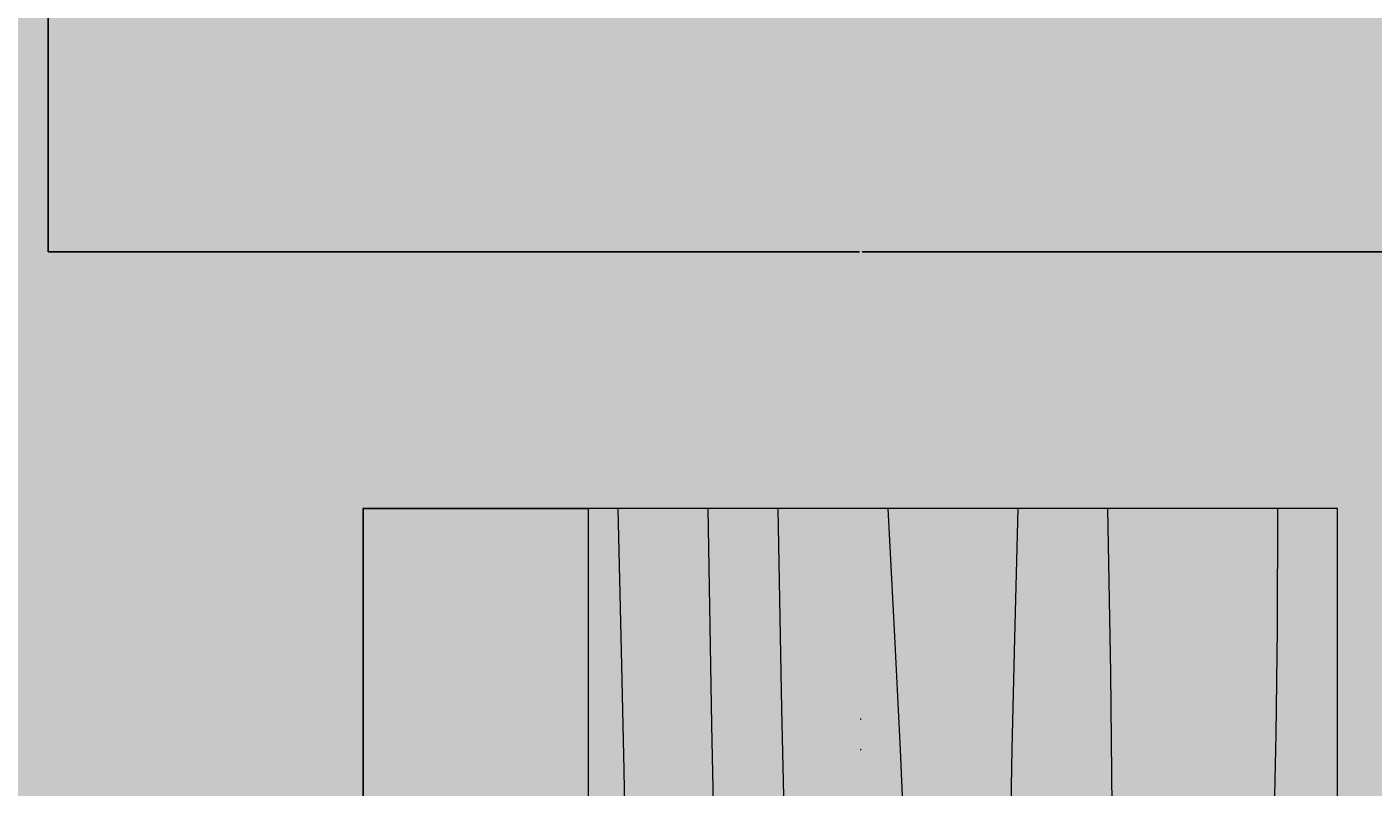
# Model space of a CAD drawing. Units: millimetres. Extents: x -229 to 16545, y -10488 to 4272.
# Tile 20 of 29: x 11572 to 12629, y -2708 to -2111. Entities that reach past the tile are written whole.
import ezdxf

# ---------------------------------------------------------------- set-up
doc = ezdxf.new("R2010")
doc.units = ezdxf.units.MM
for name, color, linetype, lineweight in [('A-ANNO-DIMS', 2, 'Continuous', 18), ('A-FURN', 8, 'Continuous', 18), ('A-FURN-PATT', 252, 'Continuous', 13)]:
    doc.layers.add(name, color=color, linetype=linetype, lineweight=lineweight)
doc.layers.add('A-FLOR-PATT', color=254, linetype='Continuous', lineweight=13, true_color=0xfeeab9)
doc.styles.get("Standard").update_dxf_attribs({"font": 'arial.ttf'})
doc.dimstyles.get("Standard").update_dxf_attribs({"dimtxt": 0.18, "dimasz": 0.18, "dimexe": 0.18, "dimexo": 0.0625, "dimgap": 0.09, "dimtad": 0, "dimtih": 1, "dimtoh": 1, "dimdec": 4, "dimzin": 0, "dimdsep": 46, "dimtxsty": 'Standard', "dimcen": 0.09, "dimadec": 0, "dimazin": 0, "dimtfac": 1, "dimtdec": 4, "dimtofl": 0, "dimtmove": 0, "dimatfit": 3, "dimfxl": 1, "dimtolj": 1, "dimtzin": 0, "dimarcsym": 0})

# ---------------------------------------------------------------- blocks, each defined once
blk = doc.blocks.new('Table - Rectangular Woodgrain 60 x 30 in.')
for p, q in [((0, 0), (0, -30)), ((60, 0), (0, 0)), ((0, -30), (60, -30))]:
    blk.add_line(p, q)
for points in [[(0, -2.4), (4.8155, -2.418), (9.0302, -2.4688), (12.709, -2.5477)], [(0, -9.2), (6.5759, -9.0858), (11.9385, -9.0365)], [(0, -12.8), (5.1847, -12.9322), (9.6213, -13.0323), (13.3963, -13.1059)], [(0, -18), (5.124, -17.7273), (9.6609, -17.5057), (13.6705, -17.3303)], [(0, -22.4), (8.0098, -22.2501), (14.4094, -22.1011)], [(0, -25.2), (8.6355, -25.0504), (15.7026, -24.9031)], [(0, -28.8), (5.6867, -28.6681), (10.45, -28.5698), (14.407, -28.5012)]]:
    blk.add_lwpolyline(points)
blk = doc.blocks.new('*D39')
at = {"layer": 'A-ANNO-DIMS', "color": 0, "lineweight": -2, "transparency": 16777216}
for p, q in [((11588.8, -2096.3), (11588.8, -2287.9)), ((12864.9, -2096.3), (12864.9, -2287.9)), ((11588.9, -2287.7), (12225.8, -2287.7)), ((12864.7, -2287.7), (12227.9, -2287.7))]:
    blk.add_line(p, q, dxfattribs=at)
at = {"layer": 'A-ANNO-DIMS', "color": 0, "transparency": 16777216}
for points in [[(11588.9, -2287.7), (11588.9, -2287.7), (11588.8, -2287.7)], [(12864.7, -2287.7), (12864.7, -2287.7), (12864.9, -2287.7)]]:
    blk.add_solid(points, dxfattribs=at)
at = {"layer": 'Defpoints', "color": 0, "transparency": 16777216}
for p in [(11588.8, -2096.3), (12864.9, -2096.3), (12864.9, -2287.7)]:
    blk.add_point(p, dxfattribs=at)
at = {"layer": 'A-ANNO-DIMS', "color": 0, "transparency": 16777216, "insert": (12226.8, -2287.7), "char_height": 0.18, "attachment_point": 5}
blk.add_mtext('\\A1;LOVESEAT 1276', dxfattribs=at)
blk = doc.blocks.new('*D41')
at = {"layer": 'A-ANNO-DIMS', "color": 0, "lineweight": -2, "transparency": 16777216}
for p, q in [((12012.6, -2489.4), (11836, -2489.4)), ((11836.2, -2489.6), (11836.2, -3077.5)), ((11836.2, -3665.8), (11836.2, -3077.9)), ((12012.6, -3666), (11836, -3666))]:
    blk.add_line(p, q, dxfattribs=at)
at = {"layer": 'A-ANNO-DIMS', "color": 0, "transparency": 16777216}
for points in [[(11836.2, -2489.6), (11836.2, -2489.6), (11836.2, -2489.4)], [(11836.2, -3665.8), (11836.2, -3665.8), (11836.2, -3666)]]:
    blk.add_solid(points, dxfattribs=at)
at = {"layer": 'Defpoints', "color": 0, "transparency": 16777216}
for p in [(12012.7, -2489.4), (11836.2, -3666), (12012.7, -3666)]:
    blk.add_point(p, dxfattribs=at)
at = {"layer": 'A-ANNO-DIMS', "color": 0, "transparency": 16777216, "insert": (11836.2, -3077.7), "char_height": 0.18, "attachment_point": 5}
blk.add_mtext('\\A1;LOW TABLE 1177', dxfattribs=at)
blk = doc.blocks.new('*D103')
at = {"layer": 'A-ANNO-DIMS', "color": 0, "lineweight": -2, "transparency": 16777216}
for p, q in [((12227, -604.2), (12226.8, -604.2)), ((12226.8, -604.2), (12226.8, -1372.9)), ((12226.7, -2654.6), (12226.9, -2654.6)), ((12226.8, -2654.7), (12226.8, -2654.5))]:
    blk.add_line(p, q, dxfattribs=at)
at = {"layer": 'A-ANNO-DIMS', "color": 0, "transparency": 16777216}
blk.add_solid([(12226.8, -1372.9), (12226.9, -1372.9), (12226.8, -1373.1)], dxfattribs=at)
at = {"layer": 'Defpoints', "color": 0, "transparency": 16777216}
for p in [(12226.8, -1373.1), (12226.8, -2654.6)]:
    blk.add_point(p, dxfattribs=at)
at = {"layer": 'A-ANNO-DIMS', "color": 0, "transparency": 16777216, "insert": (12227.6, -604.2), "char_height": 0.18, "attachment_point": 5}
blk.add_mtext('\\A1;R1281.5', dxfattribs=at)
blk = doc.blocks.new('*D104')
at = {"layer": 'A-ANNO-DIMS', "color": 0, "lineweight": -2, "transparency": 16777216}
for p, q in [((12227, -793.9), (12226.8, -793.9)), ((12226.8, -793.9), (12226.8, -1500.5)), ((12226.7, -2678.7), (12226.9, -2678.7)), ((12226.8, -2678.8), (12226.8, -2678.6))]:
    blk.add_line(p, q, dxfattribs=at)
at = {"layer": 'A-ANNO-DIMS', "color": 0, "transparency": 16777216}
blk.add_solid([(12226.8, -1500.5), (12226.9, -1500.5), (12226.8, -1500.7)], dxfattribs=at)
at = {"layer": 'Defpoints', "color": 0, "transparency": 16777216}
for p in [(12226.8, -1500.7), (12226.8, -2678.7)]:
    blk.add_point(p, dxfattribs=at)
at = {"layer": 'A-ANNO-DIMS', "color": 0, "transparency": 16777216, "insert": (12227.5, -793.9), "char_height": 0.18, "attachment_point": 5}
blk.add_mtext('\\A1;R1178', dxfattribs=at)

msp = doc.modelspace()

# ---------------------------------------------------------------- hatches: boundary and pattern name
at = {"layer": 'A-FLOR-PATT', "transparency": 33554592}
h = msp.add_hatch(color=256, dxfattribs=at)
h.dxf.hatch_style = 1
h.paths.add_polyline_path([(7975.933, -5325.772), (7943.121, -5325.772), (7943.121, -4576.49, 0.40145271), (7225.933, -5325.772, 0.40145271), (6508.746, -4576.49), (6508.746, -5325.772), (6475.933, -5325.772), (6475.933, -5438.272), (5975.933, -5438.272), (5975.933, -7267.724), (5975.933, -7438.272), (6478.619, -7438.272), (6463.448, -7355.919), (6464.88, -7356.837), (6463.849, -7358.097), (6478.619, -7438.272), (6610.327, -7438.272), (6632.656, -7409.564), (6632.525, -7406.967), (6634.208, -7407.569), (6619.273, -7426.77), (6654.466, -7438.272), (7610.517, -7438.272), (7607.41, -7421.409), (7608.842, -7422.327), (7607.812, -7423.587), (7610.517, -7438.272), (7975.933, -7438.272)])
h.paths.add_polyline_path([(13785.933, -1208.272), (9555.933, -1208.272), (9555.933, -961.785), (9705.933, -961.785), (9705.933, -918.035), (10704.976, -918.035, 0.40145271), (9705.933, 38.215), (9555.933, 38.215), (9555.933, 2021.728), (5975.933, 2021.728), (5975.933, 755.492), (5745.933, 755.492), (5745.933, 1427.266), (2918.813, 1427.266), (2918.813, -492.942), (5013.319, -492.942), (5013.319, -978.272), (5745.933, -978.272), (5745.933, -397.513), (5975.933, -397.513), (5975.933, -1208.272), (4560.933, -1208.272), (4560.933, -1265.772), (4448.433, -1265.772), (4448.433, -1298.585), (4445.933, -1298.585), (3699.151, -1298.585, 0.40145271), (4448.433, -2015.772), (4560.933, -2015.772), (4560.933, -2384.177), (5745.933, -2384.177), (5799.402, -2384.177), (5799.402, -4518.272), (5975.933, -4518.272), (5975.933, -5208.272), (6475.933, -5208.272), (6475.933, -4575.772), (6508.746, -4575.772), (6508.746, -4576.49, -0.35647263), (7216.672, -5208.272), (7235.194, -5208.272, -0.35647263), (7943.121, -4576.49), (7943.121, -4575.772), (7975.933, -4575.772), (7975.933, -5208.272), (11176.247, -5208.272), (11159.44, -5191.465), (10520.768, -5191.465), (10520.768, -4888.936), (10571.19, -4888.936), (10571.19, -4872.129), (10772.876, -4872.129), (10772.876, -4888.936), (10789.683, -4888.936), (10789.683, -4872.129), (10991.368, -4872.129), (10991.368, -4888.936), (11041.79, -4888.936), (11041.79, -4872.129), (11058.597, -4872.129, -0.09090909), (11428.354, -4872.129), (11445.162, -4872.129), (11445.162, -4888.936), (11529.197, -4888.936), (11529.197, -5191.465), (11327.512, -5191.465), (11310.704, -5208.272), (13785.933, -5208.272)])
h.paths.add_polyline_path([(11047.216, -1630.944, -1), (11402.816, -1630.944, -1)], flags=16)
h.paths.add_polyline_path([(11148.816, -1630.944), (11225.016, -1554.744), (11301.216, -1630.944), (11225.016, -1707.144)], flags=0)
h.paths.add_polyline_path([(11199.616, -1630.944, -1), (11250.416, -1630.944, -1)], flags=0)
h.paths.add_polyline_path([(11588.751, -2096.259), (11588.751, -1543.254, -0.26666697), (12864.918, -1543.254), (12864.918, -2096.259), (12737.302, -2096.259), (12737.302, -2063.121), (11716.368, -2063.121), (11716.368, -2096.259)], flags=16)
h.paths.add_polyline_path([(12012.696, -2489.42), (12600.997, -2489.42), (12600.997, -3666.022), (12012.696, -3666.022)], flags=16)
h.paths.add_polyline_path([(12176.41, -3599.403), (12174.938, -3609.076), (12173.789, -3618.819), (12173.09, -3628.559), (12172.973, -3638.221), (12173.89, -3652.852), (12175.008, -3657.025), (12172.909, -3643.473), (12173.142, -3624.297), (12175.386, -3605.273)], flags=0)
h.paths.add_polyline_path([(8026.289, -286.944), (7737.703, -287.19), (7734.87, -269.156), (8029.092, -268.905)], flags=16)
h.paths.add_polyline_path([(7733.453, -260.139), (7710.784, -115.865), (7557.191, -115.996), (7556.999, 109.744), (7412.687, 132.166), (7412.433, 429.206), (7556.707, 451.876), (7556.568, 614.769), (7412.256, 637.19), (7412.003, 934.231), (7556.276, 956.9), (7556.084, 1182.639), (7709.677, 1182.77), (7732.099, 1327.082), (8029.14, 1327.335), (8051.808, 1183.062), (8205.401, 1183.192), (8205.594, 957.454), (8349.906, 935.031), (8350.159, 637.99), (8205.885, 615.322), (8206.024, 452.43), (8350.336, 430.006), (8350.59, 132.965), (8206.316, 110.298), (8206.509, -115.442), (8052.916, -115.573), (8030.493, -259.885)], flags=16)
h.paths.add_polyline_path([(12261.416, -3475.554), (12262.632, -3486.776), (12264.032, -3497.007), (12265.554, -3506.365), (12267.136, -3514.968), (12268.719, -3522.935), (12271.304, -3535.59), (12273.606, -3548.078), (12275.271, -3561.064), (12275.93, -3574.938), (12275.325, -3590.3), (12273.425, -3607.964), (12270.795, -3625.658), (12268.066, -3641.063), (12266.318, -3649.679), (12265.456, -3653.626), (12263.984, -3659.846), (12264.032, -3659.566), (12264.342, -3658.241), (12264.807, -3656.37), (12265.456, -3653.626), (12266.318, -3649.679), (12267.409, -3644.302), (12268.668, -3637.664), (12270.019, -3630.037), (12271.384, -3621.695), (12272.69, -3612.908), (12273.857, -3603.948), (12274.81, -3595.088), (12275.47, -3586.601), (12275.782, -3578.689), (12275.757, -3571.292), (12275.423, -3564.275), (12274.816, -3557.512), (12273.964, -3550.872), (12272.896, -3544.224), (12271.645, -3537.439), (12270.24, -3530.385), (12267.543, -3517.181), (12264.612, -3501.247), (12261.849, -3481.059)], flags=0)
h.paths.add_polyline_path([(12332.136, -3408.03), (12333.483, -3416.79), (12335.077, -3424.54), (12336.915, -3431.355), (12338.991, -3437.32), (12341.266, -3442.55), (12343.694, -3447.166), (12346.229, -3451.292), (12348.826, -3455.051), (12351.438, -3458.563), (12357.476, -3466.491), (12363.61, -3476.575), (12368.309, -3489.762), (12369.929, -3503.427), (12369.842, -3516.511), (12368.43, -3530.867), (12365.816, -3545.835), (12362.382, -3559.786), (12360.968, -3564.487), (12363.063, -3557.021), (12364.898, -3549.566), (12366.473, -3542.077), (12367.773, -3534.631), (12368.781, -3527.301), (12369.483, -3520.162), (12369.863, -3513.291), (12369.906, -3506.759), (12369.599, -3500.643), (12368.93, -3494.999), (12367.924, -3489.796), (12366.61, -3484.994), (12365.024, -3480.542), (12363.19, -3476.399), (12361.141, -3472.516), (12358.909, -3468.847), (12356.525, -3465.347), (12354.02, -3461.954), (12351.438, -3458.563), (12345.462, -3450.529), (12339.923, -3439.996), (12335.85, -3428.296), (12332.68, -3412.888)], flags=0)
h.paths.add_polyline_path([(12385.287, -3334.612), (12384.977, -3342.409), (12385.02, -3349.196), (12385.4, -3355.066), (12386.104, -3360.105), (12387.112, -3364.41), (12388.412, -3368.071), (12389.987, -3371.181), (12391.823, -3373.832), (12393.919, -3376.097), (12396.337, -3377.978), (12399.153, -3379.462), (12402.445, -3380.531), (12406.289, -3381.172), (12410.758, -3381.371), (12415.935, -3381.106), (12421.893, -3380.368), (12428.658, -3379.159), (12436.069, -3377.55), (12443.907, -3375.635), (12451.961, -3373.505), (12460.015, -3371.254), (12467.853, -3368.971), (12475.263, -3366.749), (12482.029, -3364.68), (12491.877, -3361.657), (12497.701, -3360.107), (12501.639, -3359.288), (12510.135, -3358.326), (12519.662, -3365.412), (12524.243, -3378.911), (12523.764, -3390.7), (12520.746, -3401.577), (12514.248, -3415.634), (12511.518, -3420.418), (12515.856, -3412.154), (12519.153, -3405.024), (12521.516, -3398.804), (12523.049, -3393.276), (12523.865, -3388.212), (12524.059, -3383.441), (12523.7, -3378.958), (12522.853, -3374.815), (12521.576, -3371.054), (12519.931, -3367.722), (12517.982, -3364.865), (12515.786, -3362.529), (12513.405, -3360.758), (12510.877, -3359.588), (12508.136, -3358.982), (12505.086, -3358.897), (12501.639, -3359.288), (12497.701, -3360.107), (12493.183, -3361.309), (12487.988, -3362.851), (12476.403, -3366.408), (12463.335, -3370.326), (12447.372, -3374.788), (12431.759, -3378.604), (12418.504, -3380.974), (12405.811, -3381.624), (12394.725, -3378.025), (12388.039, -3368.367), (12385.583, -3357.877), (12384.826, -3346.204), (12385.428, -3331.059), (12385.953, -3325.719)], flags=0)
h.paths.add_polyline_path([(7880.016, 1173.969), (7880.373, 1175.495), (7880.433, 1175.851), (7879.484, 1171.818)], flags=0)
h.paths.add_polyline_path([(7802.33, 874.962), (7800.771, 885.032), (7798.932, 893.941), (7796.811, 901.774), (7794.419, 908.63), (7791.798, 914.639), (7789.002, 919.945), (7786.083, 924.686), (7783.093, 929.005), (7780.087, 933.043), (7774.996, 939.717), (7768.406, 949.37), (7762.174, 963.427), (7759.342, 978.002), (7758.629, 991.888), (7759.492, 1007.928), (7761.801, 1025.496), (7765.392, 1044.035), (7766.625, 1049.048), (7764.522, 1039.543), (7762.719, 1030.232), (7761.232, 1021.168), (7760.08, 1012.405), (7759.28, 1003.994), (7758.849, 995.988), (7758.806, 988.44), (7759.167, 981.404), (7759.942, 974.914), (7761.104, 968.936), (7762.617, 963.414), (7764.448, 958.299), (7766.559, 953.535), (7768.918, 949.073), (7771.487, 944.856), (7774.232, 940.835), (7777.115, 936.938), (7782.377, 930.041), (7787.845, 922.139), (7793.348, 911.698), (7798.042, 898.247), (7801.702, 880.527)], flags=0)
h.paths.add_polyline_path([(12519.068, -3228.534), (12519.615, -3236.235), (12520.529, -3242.343), (12521.78, -3247.103), (12523.337, -3250.758), (12525.171, -3253.556), (12527.248, -3255.709), (12529.522, -3257.296), (12531.95, -3258.361), (12534.486, -3258.949), (12537.082, -3259.11), (12539.694, -3258.888), (12542.277, -3258.329), (12544.781, -3257.478), (12547.173, -3256.388), (12549.46, -3255.129), (12550.455, -3254.517), (12555.825, -3251.109), (12557.835, -3249.942), (12565.181, -3246.404), (12574.565, -3253.032), (12576.931, -3265.022), (12576.627, -3277.425), (12575.416, -3290.819), (12574.851, -3295.392), (12575.708, -3287.593), (12576.322, -3280.806), (12576.688, -3274.939), (12576.812, -3269.899), (12576.688, -3265.593), (12576.322, -3261.932), (12575.708, -3258.822), (12574.851, -3256.172), (12573.753, -3253.905), (12572.439, -3252.005), (12570.943, -3250.474), (12569.293, -3249.309), (12567.523, -3248.513), (12565.658, -3248.083), (12563.732, -3248.022), (12561.777, -3248.328), (12559.814, -3248.989), (12557.835, -3249.942), (12555.825, -3251.109), (12553.77, -3252.413), (12551.652, -3253.78), (12549.46, -3255.129), (12543.167, -3258.594), (12532.661, -3259.485), (12524.685, -3253.923), (12520.949, -3245.152), (12519.138, -3233.042)], flags=0)
h.paths.add_polyline_path([(7741.293, 790.501), (7741.641, 799.467), (7741.584, 807.269), (7741.141, 814.015), (7740.329, 819.809), (7739.165, 824.757), (7737.667, 828.966), (7735.853, 832.541), (7733.74, 835.586), (7731.348, 838.188), (7728.71, 840.348), (7725.861, 842.052), (7722.836, 843.28), (7719.671, 844.015), (7716.4, 844.237), (7713.06, 843.932), (7709.684, 843.081), (7706.304, 841.686), (7702.923, 839.834), (7699.543, 837.629), (7696.164, 835.178), (7692.784, 832.585), (7684.718, 826.315), (7675.609, 820.63), (7664.001, 817.274), (7654.105, 821.884), (7647.171, 832.02), (7644.191, 846.522), (7646.321, 860.288), (7647.49, 864.223), (7645.946, 857.865), (7645.046, 852.044), (7644.827, 846.557), (7645.243, 841.404), (7646.221, 836.642), (7647.693, 832.318), (7649.587, 828.489), (7651.832, 825.206), (7654.359, 822.523), (7657.097, 820.49), (7659.984, 819.145), (7662.993, 818.452), (7666.108, 818.357), (7669.311, 818.809), (7672.583, 819.755), (7675.908, 821.139), (7679.268, 822.913), (7682.645, 825.021), (7686.025, 827.401), (7689.404, 829.958), (7692.784, 832.585), (7700.505, 838.509), (7709.871, 843.64), (7721.436, 844.698), (7733.277, 837.617), (7739.571, 825.214), (7741.557, 811.049), (7741.669, 795.575)], flags=0)
h.paths.add_polyline_path([(8377.641, 137.216), (8359.607, 134.382), (8359.356, 428.605), (8377.395, 425.802)], flags=16)
h.paths.add_polyline_path([(7650.715, 668.465), (7650.08, 677.319), (7649.023, 684.34), (7647.579, 689.811), (7645.785, 694.012), (7643.675, 697.228), (7641.286, 699.7), (7638.669, 701.521), (7635.876, 702.744), (7632.96, 703.419), (7629.974, 703.601), (7626.971, 703.344), (7624.004, 702.697), (7621.125, 701.717), (7618.375, 700.462), (7615.749, 699.013), (7614.561, 698.279), (7608.435, 694.382), (7606.125, 693.04), (7598.981, 689.594), (7589.669, 693.773), (7585.26, 702.856), (7584.221, 713.11), (7584.49, 724.584), (7585.863, 739.937), (7586.518, 745.277), (7585.539, 736.31), (7584.841, 728.507), (7584.424, 721.761), (7584.288, 715.966), (7584.433, 711.016), (7584.86, 706.807), (7585.567, 703.231), (7586.556, 700.186), (7587.821, 697.58), (7589.332, 695.397), (7591.053, 693.637), (7592.951, 692.3), (7594.989, 691.385), (7597.132, 690.895), (7599.346, 690.826), (7601.594, 691.18), (7603.851, 691.943), (7606.125, 693.04), (7608.435, 694.382), (7610.797, 695.885), (7613.229, 697.458), (7620.475, 701.929), (7632.001, 704.44), (7643.476, 699.417), (7648.536, 687.571), (7650.63, 673.661)], flags=0)
h.paths.add_polyline_path([(7385.628, 136.37), (7385.382, 424.956), (7403.416, 427.789), (7403.667, 133.567)], flags=16)
h.paths.add_polyline_path([(12993.884, -2257.186), (12959.588, -2257.186), (12959.588, -2125.099), (13531.966, -2125.099, -0.19047621), (13531.966, -3974.321), (12959.588, -3974.321), (12959.588, -3842.233), (12993.884, -3842.233)], flags=16)
h.paths.add_polyline_path([(13413.486, -3313.884), (13413.486, -2785.535), (13562.885, -2785.535, -0.04962821), (13562.885, -3313.884)], flags=0)
h.paths.add_polyline_path([(8377.21, 642.241), (8359.176, 639.407), (8358.925, 933.629), (8376.964, 930.826)], flags=16)
h.paths.add_polyline_path([(13086.058, -1864.83), (13086.058, -1449.84), (13501.048, -1449.84), (13501.048, -1864.83)], flags=16)
h.paths.add_polyline_path([(13305.814, -1862.197), (13302.103, -1859.624), (13298.088, -1857.068), (13293.799, -1854.536), (13289.262, -1852.031), (13284.504, -1849.559), (13279.554, -1847.125), (13274.439, -1844.735), (13269.17, -1842.389), (13263.701, -1840.081), (13257.97, -1837.797), (13251.914, -1835.525), (13245.472, -1833.252), (13238.582, -1830.968), (13231.18, -1828.66), (13223.206, -1826.315), (13209.182, -1822.458), (13204.584, -1821.48), (13217.962, -1824.773), (13235.072, -1829.804), (13248.777, -1834.349), (13260.829, -1838.869), (13274.479, -1844.63), (13289.675, -1852.101), (13302.553, -1859.704)], flags=0)
h.paths.add_polyline_path([(13428.104, -1820.994), (13419.007, -1818.141), (13409.95, -1815.4), (13400.766, -1812.747), (13391.271, -1810.151), (13376.087, -1806.251), (13370.618, -1805.019), (13386.304, -1808.794), (13405.087, -1813.928), (13423.014, -1819.354)], flags=0)
h.paths.add_polyline_path([(7385.197, 641.395), (7384.951, 929.98), (7402.986, 932.814), (7403.236, 638.592)], flags=16)
h.paths.add_polyline_path([(13262.537, -1725.526), (13253.246, -1724.74), (13244.516, -1724.117), (13235.94, -1723.625), (13223.267, -1723.062), (13217.598, -1722.912), (13231.966, -1723.397), (13248.733, -1724.359), (13266.899, -1725.895), (13272.802, -1726.502)], flags=0)
h.paths.add_polyline_path([(13191.893, -1641.137), (13208.675, -1640.506), (13214.057, -1640.258), (13197.763, -1640.936)], flags=0)
h.paths.add_polyline_path([(13097.524, -1608.457), (13114.284, -1609.031), (13120.126, -1609.105), (13103.045, -1608.71)], flags=0)
h.paths.add_polyline_path([(13465.328, -1521.577), (13473.906, -1517.015), (13481.761, -1511.636), (13492.562, -1502.076), (13495.327, -1497.933), (13485.818, -1508.858), (13470.208, -1519.547)], flags=0)
h.paths.add_polyline_path([(13175.015, -1500.891), (13184.046, -1501.807), (13192.721, -1502.52), (13201.114, -1503.034), (13209.273, -1503.351), (13217.244, -1503.476), (13225.078, -1503.41), (13232.821, -1503.16), (13240.524, -1502.728), (13248.233, -1502.117), (13255.993, -1501.322), (13263.825, -1500.293), (13271.746, -1498.974), (13279.775, -1497.305), (13287.928, -1495.229), (13296.222, -1492.688), (13304.675, -1489.622), (13313.304, -1485.975), (13322.089, -1481.727), (13330.859, -1477.028), (13339.408, -1472.063), (13347.526, -1467.02), (13355.006, -1462.087), (13364.86, -1455.202), (13367.224, -1453.299), (13358.544, -1459.754), (13343.348, -1469.775), (13326.143, -1479.767), (13309.023, -1488.045), (13292.249, -1494.129), (13276.009, -1498.264), (13260.299, -1500.88), (13244.401, -1502.51), (13228.945, -1503.378), (13213.316, -1503.508), (13197.047, -1502.876), (13180.088, -1501.481)], flags=0)
h.paths.add_polyline_path([(7733.501, 1336.101), (7736.303, 1354.14), (8024.889, 1354.386), (8027.723, 1336.352)], flags=16)
at = {"layer": 'A-FURN-PATT', "transparency": 33554569}
h = msp.add_hatch(color=256, dxfattribs=at)
h.dxf.hatch_style = 1
h.paths.add_polyline_path([(12600.997, -2489.42), (12553.933, -2489.42), (12553.58, -2583.852), (12552.584, -2666.503), (12551.036, -2738.644), (12549.03, -2801.547), (12546.656, -2856.483), (12544.004, -2904.723), (12541.171, -2947.542), (12538.245, -2986.207), (12535.313, -3021.787), (12532.444, -3054.526), (12529.695, -3084.461), (12527.132, -3111.629), (12524.814, -3136.073), (12522.802, -3157.826), (12521.157, -3176.928), (12519.941, -3193.42), (12519.202, -3207.371), (12518.921, -3218.994), (12519.068, -3228.534), (12519.615, -3236.235), (12520.529, -3242.343), (12521.78, -3247.103), (12523.337, -3250.758), (12525.171, -3253.556), (12527.248, -3255.709), (12529.522, -3257.296), (12531.95, -3258.361), (12534.486, -3258.949), (12537.082, -3259.11), (12539.694, -3258.888), (12542.277, -3258.329), (12544.781, -3257.478), (12547.173, -3256.388), (12549.46, -3255.129), (12551.652, -3253.78), (12559.563, -3248.675), (12566.794, -3247.543), (12572.687, -3251.706), (12575.978, -3258.498), (12576.872, -3267.431), (12576.627, -3277.425), (12575.708, -3287.593), (12574.851, -3295.392), (12573.749, -3304.309), (12572.419, -3314.522), (12570.874, -3326.221), (12569.131, -3339.597), (12567.203, -3354.842), (12565.107, -3372.146), (12562.857, -3391.705), (12560.469, -3413.705), (12557.959, -3438.275), (12555.343, -3465.264), (12552.633, -3494.46), (12549.848, -3525.645), (12547.001, -3558.61), (12544.106, -3593.137), (12541.184, -3629.012), (12538.245, -3666.022), (12600.997, -3666.022)])
h.paths.add_polyline_path([(12544.004, -2904.723), (12546.656, -2856.483), (12549.03, -2801.547), (12551.036, -2738.644), (12552.584, -2666.503), (12553.58, -2583.852), (12553.933, -2489.42), (12420.585, -2489.42), (12422.824, -2618.374), (12423.791, -2723.534), (12423.687, -2808.136), (12422.708, -2875.41), (12421.057, -2928.591), (12418.93, -2970.907), (12416.527, -3005.595), (12414.049, -3035.885), (12411.656, -3064.467), (12409.37, -3091.846), (12407.177, -3117.984), (12405.059, -3142.842), (12403.004, -3166.384), (12400.994, -3188.569), (12399.016, -3209.359), (12397.053, -3228.718), (12395.1, -3246.62), (12393.191, -3263.097), (12391.376, -3278.194), (12389.699, -3291.961), (12388.205, -3304.438), (12386.942, -3315.677), (12385.953, -3325.719), (12385.287, -3334.612), (12384.977, -3342.409), (12385.02, -3349.196), (12385.4, -3355.066), (12386.104, -3360.105), (12387.112, -3364.41), (12388.412, -3368.071), (12389.987, -3371.181), (12391.823, -3373.832), (12393.919, -3376.097), (12396.337, -3377.978), (12399.153, -3379.462), (12402.445, -3380.531), (12406.289, -3381.172), (12410.758, -3381.371), (12415.935, -3381.106), (12421.893, -3380.368), (12428.658, -3379.159), (12436.069, -3377.55), (12443.907, -3375.635), (12451.961, -3373.505), (12460.015, -3371.254), (12467.853, -3368.971), (12475.263, -3366.749), (12482.029, -3364.68), (12491.877, -3361.657), (12502.516, -3358.826), (12511.128, -3359.064), (12517.01, -3363.44), (12520.955, -3369.223), (12523.527, -3376.802), (12524.25, -3385.824), (12522.632, -3395.865), (12519.153, -3405.024), (12515.856, -3412.154), (12511.518, -3420.418), (12506.031, -3430.037), (12499.288, -3441.236), (12491.181, -3454.234), (12481.682, -3469.286), (12471.081, -3486.774), (12459.744, -3507.112), (12448.039, -3530.713), (12436.334, -3557.99), (12424.997, -3589.358), (12414.396, -3625.231), (12404.897, -3666.022), (12538.245, -3666.022), (12541.184, -3629.012), (12544.106, -3593.137), (12547.001, -3558.61), (12549.848, -3525.645), (12552.633, -3494.46), (12555.343, -3465.264), (12557.959, -3438.275), (12560.469, -3413.705), (12562.857, -3391.705), (12565.107, -3372.146), (12567.203, -3354.842), (12569.131, -3339.597), (12570.874, -3326.221), (12572.419, -3314.522), (12573.749, -3304.309), (12574.851, -3295.392), (12575.708, -3287.593), (12576.322, -3280.806), (12576.688, -3274.939), (12576.812, -3269.899), (12576.688, -3265.593), (12576.322, -3261.932), (12575.708, -3258.822), (12574.851, -3256.172), (12573.753, -3253.905), (12572.439, -3252.005), (12570.943, -3250.474), (12569.293, -3249.309), (12567.523, -3248.513), (12565.658, -3248.083), (12563.732, -3248.022), (12561.777, -3248.328), (12559.814, -3248.989), (12557.835, -3249.942), (12555.825, -3251.109), (12553.77, -3252.413), (12547.19, -3256.659), (12539.533, -3259.262), (12531.64, -3258.773), (12524.685, -3253.923), (12520.949, -3245.152), (12519.615, -3236.235), (12519.068, -3228.534), (12518.921, -3218.994), (12519.202, -3207.371), (12519.941, -3193.42), (12521.157, -3176.928), (12522.802, -3157.826), (12524.814, -3136.073), (12527.132, -3111.629), (12529.695, -3084.461), (12532.444, -3054.526), (12535.313, -3021.787), (12538.245, -2986.207), (12541.171, -2947.542)])
h.paths.add_polyline_path([(12418.93, -2970.907), (12421.057, -2928.591), (12422.708, -2875.41), (12423.687, -2808.136), (12423.791, -2723.534), (12422.824, -2618.374), (12420.585, -2489.42), (12349.989, -2489.42), (12347.396, -2591.092), (12345.433, -2678.094), (12343.99, -2752.122), (12342.962, -2814.864), (12342.239, -2868.017), (12341.715, -2913.271), (12341.284, -2952.323), (12340.837, -2986.86), (12340.288, -3018.358), (12339.633, -3047.386), (12338.883, -3074.301), (12338.06, -3099.455), (12337.173, -3123.199), (12336.242, -3145.885), (12335.279, -3167.868), (12334.301, -3189.498), (12333.326, -3211.038), (12332.381, -3232.395), (12331.496, -3253.384), (12330.706, -3273.821), (12330.037, -3293.523), (12329.52, -3312.306), (12329.188, -3329.984), (12329.071, -3346.378), (12329.194, -3361.343), (12329.561, -3374.915), (12330.175, -3387.169), (12331.032, -3398.18), (12332.136, -3408.03), (12333.483, -3416.79), (12335.077, -3424.54), (12336.915, -3431.355), (12338.991, -3437.32), (12341.266, -3442.55), (12343.694, -3447.166), (12346.229, -3451.292), (12348.826, -3455.051), (12351.438, -3458.563), (12357.476, -3466.491), (12362.356, -3474.514), (12365.989, -3482.725), (12368.611, -3492.308), (12369.929, -3503.427), (12369.863, -3513.291), (12369.483, -3520.162), (12368.781, -3527.301), (12367.773, -3534.631), (12366.473, -3542.077), (12364.898, -3549.566), (12363.063, -3557.021), (12360.968, -3564.487), (12358.568, -3572.468), (12355.799, -3581.585), (12352.603, -3592.463), (12348.916, -3605.723), (12344.678, -3621.988), (12339.827, -3641.88), (12334.301, -3666.022), (12404.897, -3666.022), (12414.396, -3625.231), (12424.997, -3589.358), (12436.334, -3557.99), (12448.039, -3530.713), (12459.744, -3507.112), (12471.081, -3486.774), (12481.682, -3469.286), (12491.181, -3454.234), (12499.288, -3441.236), (12506.031, -3430.037), (12511.518, -3420.418), (12515.856, -3412.154), (12519.153, -3405.024), (12521.516, -3398.804), (12523.049, -3393.276), (12523.865, -3388.212), (12524.059, -3383.441), (12523.7, -3378.958), (12522.853, -3374.815), (12521.576, -3371.054), (12519.931, -3367.722), (12517.982, -3364.865), (12515.786, -3362.529), (12513.405, -3360.758), (12510.877, -3359.588), (12508.136, -3358.982), (12505.086, -3358.897), (12501.639, -3359.288), (12497.701, -3360.107), (12493.183, -3361.309), (12487.988, -3362.851), (12476.403, -3366.408), (12463.335, -3370.326), (12451.961, -3373.505), (12439.372, -3376.834), (12424.661, -3380.026), (12412.995, -3381.47), (12402.039, -3380.984), (12393.748, -3376.613), (12389.022, -3369.787), (12386.442, -3362.522), (12385.041, -3352.492), (12384.977, -3342.409), (12385.287, -3334.612), (12385.953, -3325.719), (12386.942, -3315.677), (12388.205, -3304.438), (12389.699, -3291.961), (12391.376, -3278.194), (12393.191, -3263.097), (12395.1, -3246.62), (12397.053, -3228.718), (12399.016, -3209.359), (12400.994, -3188.569), (12403.004, -3166.384), (12405.059, -3142.842), (12407.177, -3117.984), (12409.37, -3091.846), (12411.656, -3064.467), (12414.049, -3035.885), (12416.527, -3005.595)])
h.paths.add_polyline_path([(12340.837, -2986.86), (12341.284, -2952.323), (12341.715, -2913.271), (12342.239, -2868.017), (12342.962, -2814.864), (12343.99, -2752.122), (12345.433, -2678.094), (12347.396, -2591.092), (12349.989, -2489.42), (12248.016, -2489.42), (12253.364, -2589.902), (12257.71, -2678.871), (12261.149, -2757.499), (12263.787, -2826.958), (12265.718, -2888.42), (12267.044, -2943.055), (12267.866, -2992.039), (12268.279, -3036.54), (12268.378, -3077.58), (12268.209, -3115.572), (12267.809, -3150.776), (12267.219, -3183.452), (12266.473, -3213.86), (12265.614, -3242.261), (12264.679, -3268.917), (12263.704, -3294.084), (12262.732, -3317.981), (12261.804, -3340.639), (12260.969, -3362.039), (12260.273, -3382.167), (12259.759, -3401.008), (12259.477, -3418.547), (12259.469, -3434.769), (12259.782, -3449.659), (12260.445, -3463.221), (12261.416, -3475.554), (12262.632, -3486.776), (12264.032, -3497.007), (12265.554, -3506.365), (12267.136, -3514.968), (12268.719, -3522.935), (12271.304, -3535.59), (12273.606, -3548.078), (12275.271, -3561.064), (12275.757, -3571.292), (12275.782, -3578.689), (12275.47, -3586.601), (12274.81, -3595.088), (12273.857, -3603.948), (12272.69, -3612.908), (12271.384, -3621.695), (12270.019, -3630.037), (12268.066, -3641.063), (12265.651, -3652.97), (12264.342, -3658.241), (12264.032, -3659.566), (12263.842, -3660.678), (12263.746, -3661.906), (12263.708, -3663.576), (12263.704, -3666.022), (12334.301, -3666.022), (12339.827, -3641.88), (12344.678, -3621.988), (12348.916, -3605.723), (12352.603, -3592.463), (12355.799, -3581.585), (12358.568, -3572.468), (12360.968, -3564.487), (12363.063, -3557.021), (12364.898, -3549.566), (12366.473, -3542.077), (12367.773, -3534.631), (12368.781, -3527.301), (12369.483, -3520.162), (12369.863, -3513.291), (12369.906, -3506.759), (12369.599, -3500.643), (12368.93, -3494.999), (12367.924, -3489.796), (12366.61, -3484.994), (12365.024, -3480.542), (12363.19, -3476.399), (12361.141, -3472.516), (12358.909, -3468.847), (12356.525, -3465.347), (12354.02, -3461.954), (12347.609, -3453.536), (12342.257, -3444.828), (12337.759, -3434.488), (12335.077, -3424.54), (12333.483, -3416.79), (12332.136, -3408.03), (12331.032, -3398.18), (12330.175, -3387.169), (12329.561, -3374.915), (12329.194, -3361.343), (12329.071, -3346.378), (12329.188, -3329.984), (12329.52, -3312.306), (12330.037, -3293.523), (12330.706, -3273.821), (12331.496, -3253.384), (12332.381, -3232.395), (12333.326, -3211.038), (12334.301, -3189.498), (12335.279, -3167.868), (12336.242, -3145.885), (12337.173, -3123.199), (12338.06, -3099.455), (12338.883, -3074.301), (12339.633, -3047.386), (12340.288, -3018.358)])
h.paths.add_polyline_path([(12267.866, -2992.039), (12267.044, -2943.055), (12265.718, -2888.42), (12263.787, -2826.958), (12261.149, -2757.499), (12257.71, -2678.871), (12253.364, -2589.902), (12248.016, -2489.42), (12161.732, -2489.42), (12164.672, -2646.493), (12167.594, -2771.989), (12170.488, -2870.184), (12173.336, -2945.353), (12176.12, -3001.769), (12178.83, -3043.709), (12181.446, -3075.446), (12183.956, -3101.253), (12186.347, -3124.72), (12188.614, -3146.693), (12190.759, -3167.333), (12192.781, -3186.802), (12194.681, -3205.259), (12196.458, -3222.865), (12198.113, -3239.782), (12199.644, -3256.172), (12201.048, -3272.182), (12202.3, -3287.915), (12203.368, -3303.466), (12204.221, -3318.924), (12204.827, -3334.383), (12205.161, -3349.932), (12205.186, -3365.667), (12204.874, -3381.676), (12204.208, -3398.008), (12203.219, -3414.517), (12201.956, -3431.021), (12200.462, -3447.329), (12198.784, -3463.254), (12196.97, -3478.607), (12195.062, -3493.203), (12193.108, -3506.853), (12191.149, -3519.429), (12189.196, -3531.038), (12187.259, -3541.853), (12185.347, -3552.039), (12183.462, -3561.763), (12181.619, -3571.2), (12179.819, -3580.51), (12178.073, -3589.87), (12176.41, -3599.403), (12174.938, -3609.076), (12173.789, -3618.819), (12173.09, -3628.559), (12172.973, -3638.221), (12173.569, -3647.734), (12175.008, -3657.025), (12177.42, -3666.022), (12263.654, -3666.022), (12263.777, -3660.515), (12264.807, -3656.37), (12265.456, -3653.626), (12266.318, -3649.679), (12267.409, -3644.302), (12268.668, -3637.664), (12270.019, -3630.037), (12271.384, -3621.695), (12272.69, -3612.908), (12273.857, -3603.948), (12274.81, -3595.088), (12275.47, -3586.601), (12275.782, -3578.689), (12275.757, -3571.292), (12275.423, -3564.275), (12274.816, -3557.512), (12273.964, -3550.872), (12272.896, -3544.224), (12271.645, -3537.439), (12270.24, -3530.385), (12267.543, -3517.181), (12265.554, -3506.365), (12264.032, -3497.007), (12262.632, -3486.776), (12261.416, -3475.554), (12260.445, -3463.221), (12259.782, -3449.659), (12259.469, -3434.769), (12259.477, -3418.547), (12259.759, -3401.008), (12260.273, -3382.167), (12260.969, -3362.039), (12261.804, -3340.639), (12262.732, -3317.981), (12263.704, -3294.084), (12264.679, -3268.917), (12265.614, -3242.261), (12266.473, -3213.86), (12267.219, -3183.452), (12267.809, -3150.776), (12268.209, -3115.572), (12268.378, -3077.58), (12268.279, -3036.54)])
h.paths.add_polyline_path([(12178.83, -3043.709), (12176.12, -3001.769), (12173.336, -2945.353), (12170.488, -2870.184), (12167.594, -2771.989), (12164.672, -2646.493), (12161.732, -2489.42), (12106.824, -2489.42), (12109.758, -2658.763), (12112.646, -2797.349), (12115.441, -2909.171), (12118.1, -2998.218), (12120.575, -3068.485), (12122.818, -3123.958), (12124.787, -3168.631), (12126.434, -3206.494), (12127.727, -3240.902), (12128.682, -3272.678), (12129.331, -3302.001), (12129.703, -3329.057), (12129.831, -3354.028), (12129.742, -3377.101), (12129.472, -3398.457), (12129.048, -3418.282), (12128.499, -3436.761), (12127.832, -3454.092), (12127.062, -3470.478), (12126.189, -3486.119), (12125.224, -3501.217), (12124.177, -3515.972), (12123.052, -3530.585), (12121.857, -3545.257), (12120.61, -3560.145), (12119.355, -3575.225), (12118.147, -3590.433), (12117.037, -3605.699), (12116.082, -3620.96), (12115.331, -3636.144), (12114.843, -3651.187), (12114.668, -3666.022), (12177.42, -3666.022), (12175.008, -3657.025), (12173.569, -3647.734), (12172.973, -3638.221), (12173.09, -3628.559), (12173.789, -3618.819), (12174.938, -3609.076), (12176.41, -3599.403), (12178.073, -3589.87), (12179.819, -3580.51), (12181.619, -3571.2), (12183.462, -3561.763), (12185.347, -3552.039), (12187.259, -3541.853), (12189.196, -3531.038), (12191.149, -3519.429), (12193.108, -3506.853), (12195.062, -3493.203), (12196.97, -3478.607), (12198.784, -3463.254), (12200.462, -3447.329), (12201.956, -3431.021), (12203.219, -3414.517), (12204.208, -3398.008), (12204.874, -3381.676), (12205.186, -3365.667), (12205.161, -3349.932), (12204.827, -3334.383), (12204.221, -3318.924), (12203.368, -3303.466), (12202.3, -3287.915), (12201.048, -3272.182), (12199.644, -3256.172), (12198.113, -3239.782), (12196.458, -3222.865), (12194.681, -3205.259), (12192.781, -3186.802), (12190.759, -3167.333), (12188.614, -3146.693), (12186.347, -3124.72), (12183.956, -3101.253), (12181.446, -3075.446)])
h.paths.add_polyline_path([(12120.575, -3068.485), (12118.1, -2998.218), (12115.441, -2909.171), (12112.646, -2797.349), (12109.758, -2658.763), (12106.824, -2489.42), (12036.228, -2489.42), (12038.815, -2600.936), (12040.742, -2694.345), (12042.088, -2771.942), (12042.927, -2836.027), (12043.339, -2888.898), (12043.398, -2932.852), (12043.18, -2970.187), (12042.764, -3003.203), (12042.215, -3033.834), (12041.56, -3062.574), (12040.811, -3089.552), (12039.985, -3114.898), (12039.101, -3138.743), (12038.168, -3161.217), (12037.207, -3182.448), (12036.228, -3202.57), (12035.254, -3221.743), (12034.318, -3240.249), (12033.459, -3258.402), (12032.714, -3276.518), (12032.124, -3294.908), (12031.724, -3313.888), (12031.553, -3333.773), (12031.653, -3354.875), (12032.083, -3377.629), (12033.01, -3402.94), (12034.628, -3431.837), (12037.126, -3465.345), (12040.697, -3504.492), (12045.533, -3550.301), (12051.822, -3603.803), (12059.76, -3666.022), (12114.668, -3666.022), (12114.843, -3651.187), (12115.331, -3636.144), (12116.082, -3620.96), (12117.037, -3605.699), (12118.147, -3590.433), (12119.355, -3575.225), (12120.61, -3560.145), (12121.857, -3545.257), (12123.052, -3530.585), (12124.177, -3515.972), (12125.224, -3501.217), (12126.189, -3486.119), (12127.062, -3470.478), (12127.832, -3454.092), (12128.499, -3436.761), (12129.048, -3418.282), (12129.472, -3398.457), (12129.742, -3377.101), (12129.831, -3354.028), (12129.703, -3329.057), (12129.331, -3302.001), (12128.682, -3272.678), (12127.727, -3240.902), (12126.434, -3206.494), (12124.787, -3168.631), (12122.818, -3123.958)])
h.paths.add_polyline_path([(12042.215, -3033.834), (12042.764, -3003.203), (12043.18, -2970.187), (12043.398, -2932.852), (12043.339, -2888.898), (12042.927, -2836.027), (12042.088, -2771.942), (12040.742, -2694.345), (12038.815, -2600.936), (12036.228, -2489.42), (12012.696, -2489.42), (12012.696, -3666.022), (12059.76, -3666.022), (12051.822, -3603.803), (12045.533, -3550.301), (12040.697, -3504.492), (12037.126, -3465.345), (12034.628, -3431.837), (12033.01, -3402.94), (12032.083, -3377.629), (12031.653, -3354.875), (12031.553, -3333.773), (12031.724, -3313.888), (12032.124, -3294.908), (12032.714, -3276.518), (12033.459, -3258.402), (12034.318, -3240.249), (12035.254, -3221.743), (12036.228, -3202.57), (12037.207, -3182.448), (12038.168, -3161.217), (12039.101, -3138.743), (12039.985, -3114.898), (12040.811, -3089.552), (12041.56, -3062.574)])
h.paths.add_polyline_path([(13347.526, -1467.02), (13355.006, -1462.087), (13361.641, -1457.451), (13367.224, -1453.299), (13371.521, -1449.84), (13086.058, -1449.84), (13086.058, -1489.363), (13102.895, -1491.509), (13118.03, -1493.501), (13131.658, -1495.331), (13143.974, -1496.992), (13155.175, -1498.477), (13165.457, -1499.778), (13175.015, -1500.891), (13184.046, -1501.807), (13192.721, -1502.52), (13201.114, -1503.034), (13209.273, -1503.351), (13217.244, -1503.476), (13225.078, -1503.41), (13232.821, -1503.16), (13240.524, -1502.728), (13248.233, -1502.117), (13255.993, -1501.322), (13263.825, -1500.293), (13271.746, -1498.974), (13279.775, -1497.305), (13287.928, -1495.229), (13296.222, -1492.688), (13304.675, -1489.622), (13313.304, -1485.975), (13322.089, -1481.727), (13330.859, -1477.028), (13339.408, -1472.063)], flags=17)
h.paths.add_polyline_path([(13481.761, -1511.636), (13488.9, -1505.317), (13495.327, -1497.933), (13501.048, -1489.363), (13501.048, -1449.84), (13371.521, -1449.84), (13367.224, -1453.299), (13361.641, -1457.451), (13355.006, -1462.087), (13347.526, -1467.02), (13339.408, -1472.063), (13330.859, -1477.028), (13322.089, -1481.727), (13313.304, -1485.975), (13304.675, -1489.622), (13296.222, -1492.688), (13287.928, -1495.229), (13279.775, -1497.305), (13271.746, -1498.974), (13263.825, -1500.293), (13255.993, -1501.322), (13248.233, -1502.117), (13240.524, -1502.728), (13232.821, -1503.16), (13225.078, -1503.41), (13217.244, -1503.476), (13209.273, -1503.351), (13201.114, -1503.034), (13192.721, -1502.52), (13184.046, -1501.807), (13175.015, -1500.891), (13165.457, -1499.778), (13155.175, -1498.477), (13143.974, -1496.992), (13131.658, -1495.331), (13118.03, -1493.501), (13102.895, -1491.509), (13086.058, -1489.363), (13086.058, -1528.886), (13104.044, -1529.875), (13122.361, -1531.009), (13140.808, -1532.253), (13159.186, -1533.57), (13177.296, -1534.925), (13194.937, -1536.281), (13211.91, -1537.602), (13228.015, -1538.852), (13243.116, -1539.998), (13257.327, -1541.017), (13270.825, -1541.888), (13283.787, -1542.59), (13296.39, -1543.103), (13308.811, -1543.407), (13321.227, -1543.48), (13333.816, -1543.302), (13346.703, -1542.854), (13359.802, -1542.129), (13372.977, -1541.12), (13386.091, -1539.822), (13399.008, -1538.228), (13411.589, -1536.331), (13423.699, -1534.127), (13435.201, -1531.609), (13445.981, -1528.75), (13456.022, -1525.448), (13465.328, -1521.577), (13473.906, -1517.015)])
h.paths.add_polyline_path([(13473.169, -1576.927), (13501.048, -1568.409), (13501.048, -1489.363), (13495.327, -1497.933), (13488.9, -1505.317), (13481.761, -1511.636), (13473.906, -1517.015), (13465.328, -1521.577), (13456.022, -1525.448), (13445.981, -1528.75), (13435.201, -1531.609), (13423.699, -1534.127), (13411.589, -1536.331), (13399.008, -1538.228), (13386.091, -1539.822), (13372.977, -1541.12), (13359.802, -1542.129), (13346.703, -1542.854), (13333.816, -1543.302), (13321.227, -1543.48), (13308.811, -1543.407), (13296.39, -1543.103), (13283.787, -1542.59), (13270.825, -1541.888), (13257.327, -1541.017), (13243.116, -1539.998), (13228.015, -1538.852), (13211.91, -1537.602), (13194.937, -1536.281), (13177.296, -1534.925), (13159.186, -1533.57), (13140.808, -1532.253), (13122.361, -1531.009), (13104.044, -1529.875), (13086.058, -1528.886), (13086.058, -1607.932), (13097.524, -1608.457), (13108.847, -1608.845), (13120.126, -1609.105), (13131.46, -1609.251), (13142.948, -1609.292), (13154.691, -1609.241), (13166.786, -1609.108), (13179.335, -1608.907), (13192.433, -1608.641), (13206.166, -1608.296), (13220.617, -1607.849), (13235.868, -1607.277), (13252.002, -1606.56), (13269.102, -1605.677), (13287.251, -1604.604), (13306.532, -1603.319), (13327.007, -1601.774), (13348.658, -1599.805), (13371.445, -1597.222), (13395.329, -1593.833), (13420.269, -1589.449), (13446.229, -1583.876)])
h.paths.add_polyline_path([(13501.048, -1607.932), (13458.096, -1615.209), (13420.819, -1621.063), (13388.585, -1625.678), (13360.757, -1629.235), (13336.7, -1631.917), (13315.782, -1633.906), (13297.366, -1635.385), (13280.818, -1636.535), (13265.584, -1637.513), (13251.437, -1638.359), (13238.231, -1639.089), (13225.82, -1639.718), (13214.057, -1640.258), (13202.797, -1640.727), (13191.893, -1641.137), (13181.2, -1641.502), (13170.572, -1641.845), (13159.867, -1642.207), (13148.942, -1642.635), (13137.655, -1643.178), (13125.865, -1643.884), (13113.431, -1644.799), (13100.208, -1645.973), (13086.058, -1647.454), (13086.058, -1686.977), (13124.833, -1683.82), (13159.932, -1681.185), (13191.674, -1679.027), (13220.38, -1677.299), (13246.37, -1675.957), (13269.963, -1674.954), (13291.481, -1674.247), (13311.243, -1673.788), (13329.68, -1673.559), (13347.664, -1673.645), (13366.176, -1674.156), (13386.201, -1675.203), (13408.718, -1676.899), (13434.71, -1679.352), (13465.16, -1682.674), (13501.048, -1686.977)])
h.paths.add_polyline_path([(13501.048, -1686.977), (13465.16, -1682.674), (13434.71, -1679.352), (13408.718, -1676.899), (13386.201, -1675.203), (13366.176, -1674.156), (13347.664, -1673.645), (13329.68, -1673.559), (13311.243, -1673.788), (13291.481, -1674.247), (13269.963, -1674.954), (13246.37, -1675.957), (13220.38, -1677.299), (13191.674, -1679.027), (13159.932, -1681.185), (13124.833, -1683.82), (13086.058, -1686.977), (13086.058, -1726.5), (13102.94, -1724.807), (13119.714, -1723.593), (13136.181, -1722.793), (13152.144, -1722.337), (13167.406, -1722.161), (13181.77, -1722.195), (13195.037, -1722.374), (13207.013, -1722.63), (13217.598, -1722.912), (13227.103, -1723.233), (13235.94, -1723.625), (13244.516, -1724.117), (13253.246, -1724.74), (13262.537, -1725.526), (13272.802, -1726.502), (13284.449, -1727.701), (13297.939, -1729.184), (13313.919, -1731.151), (13333.085, -1733.832), (13356.132, -1737.458), (13383.755, -1742.259), (13416.652, -1748.466), (13455.518, -1756.31), (13501.048, -1766.023)])
h.paths.add_polyline_path([(13420.819, -1621.063), (13458.096, -1615.209), (13501.048, -1607.932), (13501.048, -1568.409), (13473.169, -1576.927), (13446.229, -1583.876), (13420.269, -1589.449), (13395.329, -1593.833), (13371.445, -1597.222), (13348.658, -1599.805), (13327.007, -1601.774), (13306.532, -1603.319), (13287.251, -1604.604), (13269.102, -1605.677), (13252.002, -1606.56), (13235.868, -1607.277), (13220.617, -1607.849), (13206.166, -1608.296), (13192.433, -1608.641), (13179.335, -1608.907), (13166.786, -1609.108), (13154.691, -1609.241), (13142.948, -1609.292), (13131.46, -1609.251), (13120.126, -1609.105), (13108.847, -1608.845), (13097.524, -1608.457), (13086.058, -1607.932), (13086.058, -1647.454), (13100.208, -1645.973), (13113.431, -1644.799), (13125.865, -1643.884), (13137.655, -1643.178), (13148.942, -1642.635), (13159.867, -1642.207), (13170.572, -1641.845), (13181.2, -1641.502), (13191.893, -1641.137), (13202.797, -1640.727), (13214.057, -1640.258), (13225.82, -1639.718), (13238.231, -1639.089), (13251.437, -1638.359), (13265.584, -1637.513), (13280.818, -1636.535), (13297.366, -1635.385), (13315.782, -1633.906), (13336.7, -1631.917), (13360.757, -1629.235), (13388.585, -1625.678)])
h.paths.add_polyline_path([(13356.132, -1737.458), (13333.085, -1733.832), (13313.919, -1731.151), (13297.939, -1729.184), (13284.449, -1727.701), (13272.802, -1726.502), (13262.537, -1725.526), (13253.246, -1724.74), (13244.516, -1724.117), (13235.94, -1723.625), (13227.103, -1723.233), (13217.598, -1722.912), (13207.013, -1722.63), (13195.037, -1722.374), (13181.77, -1722.195), (13167.406, -1722.161), (13152.144, -1722.337), (13136.181, -1722.793), (13119.714, -1723.593), (13102.94, -1724.807), (13086.058, -1726.5), (13086.058, -1766.023), (13139.44, -1771.317), (13184.365, -1776.092), (13221.843, -1780.403), (13252.878, -1784.307), (13278.478, -1787.865), (13299.651, -1791.133), (13317.401, -1794.169), (13332.737, -1797.031), (13346.528, -1799.772), (13359.094, -1802.425), (13370.618, -1805.019), (13381.282, -1807.585), (13391.271, -1810.151), (13400.766, -1812.747), (13409.95, -1815.4), (13419.007, -1818.141), (13428.104, -1820.994), (13437.348, -1823.975), (13446.831, -1827.091), (13456.644, -1830.354), (13466.882, -1833.773), (13477.633, -1837.359), (13488.991, -1841.121), (13501.048, -1845.069), (13501.048, -1766.023), (13455.518, -1756.31), (13416.652, -1748.466), (13383.755, -1742.259)])
h.paths.add_polyline_path([(13299.651, -1791.133), (13278.478, -1787.865), (13252.878, -1784.307), (13221.843, -1780.403), (13184.365, -1776.092), (13139.44, -1771.317), (13086.058, -1766.023), (13086.058, -1805.546), (13115.797, -1808.369), (13140.752, -1811.122), (13161.515, -1813.805), (13178.68, -1816.424), (13192.839, -1818.981), (13204.584, -1821.48), (13214.509, -1823.923), (13223.206, -1826.315), (13231.18, -1828.66), (13238.582, -1830.968), (13245.472, -1833.252), (13251.914, -1835.525), (13257.97, -1837.797), (13263.701, -1840.081), (13269.17, -1842.389), (13274.439, -1844.735), (13279.554, -1847.125), (13284.504, -1849.559), (13289.262, -1852.031), (13293.799, -1854.536), (13298.088, -1857.068), (13302.103, -1859.624), (13305.814, -1862.197), (13309.259, -1864.83), (13501.048, -1864.83), (13501.048, -1845.069), (13488.991, -1841.121), (13477.633, -1837.359), (13466.882, -1833.773), (13456.644, -1830.354), (13446.831, -1827.091), (13437.348, -1823.975), (13428.104, -1820.994), (13419.007, -1818.141), (13409.95, -1815.4), (13400.766, -1812.747), (13391.271, -1810.151), (13381.282, -1807.585), (13370.618, -1805.019), (13359.094, -1802.425), (13346.528, -1799.772), (13332.737, -1797.031), (13317.401, -1794.169)])
h.paths.add_polyline_path([(13245.472, -1833.252), (13238.582, -1830.968), (13231.18, -1828.66), (13223.206, -1826.315), (13214.509, -1823.923), (13204.584, -1821.48), (13192.839, -1818.981), (13178.68, -1816.424), (13161.515, -1813.805), (13140.752, -1811.122), (13115.797, -1808.369), (13086.058, -1805.546), (13086.058, -1864.83), (13309.259, -1864.83), (13305.814, -1862.197), (13302.103, -1859.624), (13298.088, -1857.068), (13293.799, -1854.536), (13289.262, -1852.031), (13284.504, -1849.559), (13279.554, -1847.125), (13274.439, -1844.735), (13269.17, -1842.389), (13263.701, -1840.081), (13257.97, -1837.797), (13251.914, -1835.525)], flags=17)

# ---------------------------------------------------------------- block references
at = {"layer": 'A-FURN', "xscale": 19.61002860704382, "yscale": 19.61002860704382, "zscale": 19.61002860704382, "rotation": 270}
msp.add_blockref('Table - Rectangular Woodgrain 60 x 30 in.', (12600.997, -2489.42), dxfattribs=at)

# ---------------------------------------------------------------- dimensions: what is measured, and where the dimension line sits
at = {"layer": 'A-ANNO-DIMS'}
for center, mpoint, override, picture, middle in [((12226.834, -2654.582), (12226.835, -1373.098), {"dimdec": 1, "dimlfac": 1, "dimrnd": 0, "dimzin": 0, "dimdsep": 46, "dimlunit": 2}, '*D103', (12227.565, -604.208)), ((12226.834, -2678.71), (12226.834, -1500.713), {"dimdec": 0, "dimlfac": 1, "dimrnd": 0, "dimzin": 0, "dimdsep": 46, "dimlunit": 2}, '*D104', (12227.459, -793.916))]:
    dim = msp.add_radius_dim(center=center, mpoint=mpoint, dimstyle='Standard', override=override, dxfattribs=at)
    dim.commit()
    dim.dimension.update_dxf_attribs({"geometry": picture, "text_midpoint": middle, "dimtype": 164})
dim = msp.add_linear_dim(base=(12864.918, -2287.684), p1=(11588.751, -2096.259), p2=(12864.918, -2096.259), text='LOVESEAT <>', dimstyle='Standard', override={"dimdec": 0, "dimlfac": 1, "dimrnd": 0, "dimzin": 0, "dimdsep": 46, "dimlunit": 2}, dxfattribs=at)
dim.commit()
dim.dimension.update_dxf_attribs({"geometry": '*D39', "text_midpoint": (12226.835, -2287.684)})
dim = msp.add_linear_dim(base=(11836.206, -3666.022), p1=(12012.696, -2489.42), p2=(12012.696, -3666.022), angle=270, text='LOW TABLE <>', dimstyle='Standard', override={"dimdec": 0, "dimlfac": 1, "dimrnd": 0, "dimzin": 0, "dimdsep": 46, "dimlunit": 2}, dxfattribs=at)
dim.commit()
dim.dimension.update_dxf_attribs({"geometry": '*D41', "text_midpoint": (11836.206, -3077.721)})

doc.saveas('drawing.dxf')
